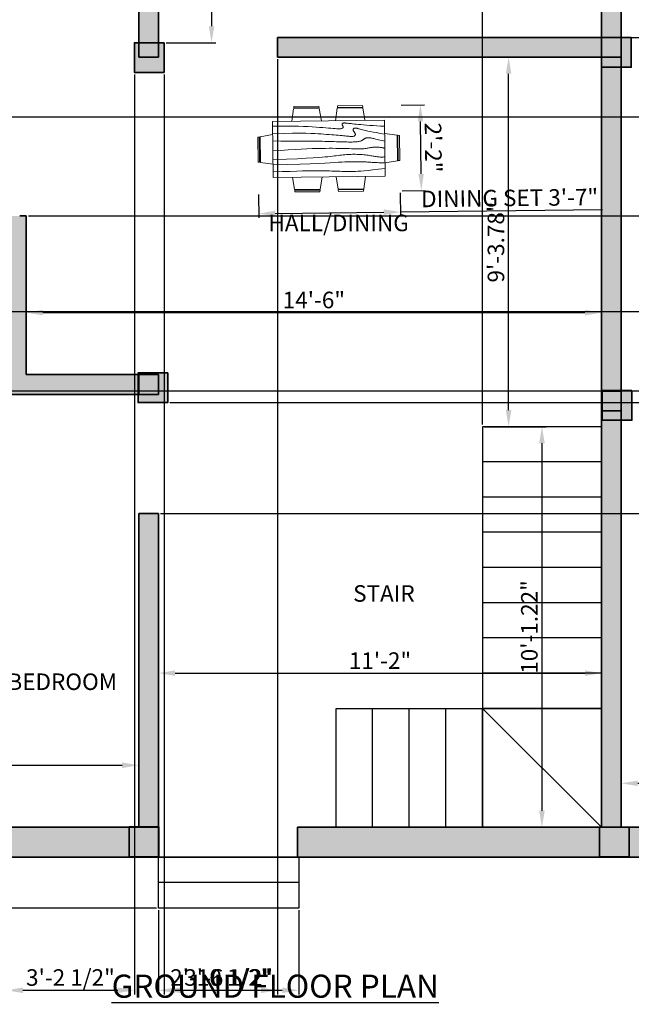
# Model space of a CAD drawing. Units: inches. Extents: x -36 to 490, y -420 to 94.
# Tile 2 of 4: x 99 to 284, y -420 to -122. Entities that reach past the tile are written whole.
import ezdxf

# ---------------------------------------------------------------- set-up
doc = ezdxf.new("R2010")
doc.units = ezdxf.units.IN
for name, color, linetype, lineweight in [('A-ANNO-DIMS', 2, 'Continuous', 18), ('A-ANNO-TEXT', 7, 'Continuous', 25), ('A-AREA-IDEN', 1, 'Continuous', 18), ('A-COLS', 1, 'Continuous', 35), ('A-FLOR-STRS', 3, 'Continuous', 25), ('A-WALL', 7, 'Continuous', 35), ('furn', 8, 'Continuous', 18)]:
    doc.layers.add(name, color=color, linetype=linetype, lineweight=lineweight)
doc.layers.add('A-WALL-PATT', color=177, linetype='Continuous', lineweight=13, true_color=0x293189)
doc.styles.get("Standard").update_dxf_attribs({"font": 'arial.ttf'})
doc.dimstyles.new('ISO-25', dxfattribs={"dimtxt": 5, "dimasz": 5, "dimexe": 1.25, "dimexo": 0.625, "dimtad": 1, "dimlunit": 3, "dimtxsty": 'Standard', "dimcen": 2.5, "dimadec": 0, "dimazin": 0, "dimtfac": 1, "dimtmove": 0, "dimatfit": 3, "dimfxl": 1, "dimarcsym": 0})

# ---------------------------------------------------------------- blocks, each defined once
blk = doc.blocks.new('*D1')
at = {"layer": 'A-ANNO-DIMS', "color": 0, "lineweight": -2, "transparency": 16777216}
for p, q in [((280.98, -352.29), (280.98, -351.67)), ((285.98, -352.92), (401.98, -352.92)), ((406.98, -352.29), (406.98, -351.67))]:
    blk.add_line(p, q, dxfattribs=at)
at = {"layer": 'A-ANNO-DIMS', "color": 0, "transparency": 16777216}
for points in [[(285.98, -352.09), (285.98, -353.75), (280.98, -352.92)], [(401.98, -352.09), (401.98, -353.75), (406.98, -352.92)]]:
    blk.add_solid(points, dxfattribs=at)
at = {"layer": 'Defpoints', "color": 0, "transparency": 16777216}
for p in [(280.98, -352.92), (406.98, -352.92), (406.98, -352.92)]:
    blk.add_point(p, dxfattribs=at)
at = {"layer": 'A-ANNO-DIMS', "color": 0, "transparency": 16777216, "insert": (343.98, -349.74), "char_height": 5, "attachment_point": 5}
blk.add_mtext('10\'-6"', dxfattribs=at)
blk = doc.blocks.new('*D3')
at = {"layer": 'A-ANNO-DIMS', "color": 0, "lineweight": -2, "transparency": 16777216}
for p, q in [((274.98, -309.55), (274.98, -320.83)), ((140.98, -319.35), (140.98, -320.83)), ((145.98, -319.58), (269.98, -319.58))]:
    blk.add_line(p, q, dxfattribs=at)
at = {"layer": 'A-ANNO-DIMS', "color": 0, "transparency": 16777216}
for points in [[(145.98, -318.74), (145.98, -320.41), (140.98, -319.58)], [(269.98, -318.74), (269.98, -320.41), (274.98, -319.58)]]:
    blk.add_solid(points, dxfattribs=at)
at = {"layer": 'Defpoints', "color": 0, "transparency": 16777216}
for p in [(274.98, -308.92), (140.98, -318.73), (274.98, -319.58)]:
    blk.add_point(p, dxfattribs=at)
at = {"layer": 'A-ANNO-DIMS', "color": 0, "transparency": 16777216, "insert": (207.98, -316.44), "char_height": 5, "attachment_point": 5}
blk.add_mtext('11\'-2"', dxfattribs=at)
blk = doc.blocks.new('*D4')
at = {"layer": 'A-ANNO-DIMS', "color": 0, "lineweight": -2, "transparency": 16777216}
for p, q in [((239.61, -245.01), (258.23, -245.01)), ((256.98, -250.01), (256.98, -361.23)), ((239.61, -366.23), (258.23, -366.23))]:
    blk.add_line(p, q, dxfattribs=at)
at = {"layer": 'A-ANNO-DIMS', "color": 0, "transparency": 16777216}
for points in [[(256.15, -250.01), (257.82, -250.01), (256.98, -245.01)], [(256.15, -361.23), (257.82, -361.23), (256.98, -366.23)]]:
    blk.add_solid(points, dxfattribs=at)
at = {"layer": 'Defpoints', "color": 0, "transparency": 16777216}
for p in [(238.98, -245.01), (238.98, -366.23), (256.98, -366.23)]:
    blk.add_point(p, dxfattribs=at)
at = {"layer": 'A-ANNO-DIMS', "color": 0, "transparency": 16777216, "insert": (253.81, -305.62), "char_height": 5, "attachment_point": 5, "rotation": 90}
blk.add_mtext('10\'-1.22"', dxfattribs=at)
blk = doc.blocks.new('*D5')
at = {"layer": 'A-ANNO-DIMS', "color": 0, "lineweight": -2, "transparency": 16777216}
for p, q in [((9.59, -330.42), (9.59, -348.7)), ((134.98, -330.42), (134.98, -348.7)), ((14.59, -347.45), (129.98, -347.45))]:
    blk.add_line(p, q, dxfattribs=at)
at = {"layer": 'A-ANNO-DIMS', "color": 0, "transparency": 16777216}
for points in [[(14.59, -346.62), (14.59, -348.29), (9.59, -347.45)], [(129.98, -346.62), (129.98, -348.29), (134.98, -347.45)]]:
    blk.add_solid(points, dxfattribs=at)
at = {"layer": 'Defpoints', "color": 0, "transparency": 16777216}
for p in [(9.59, -329.79), (134.98, -329.79), (134.98, -347.45)]:
    blk.add_point(p, dxfattribs=at)
at = {"layer": 'A-ANNO-DIMS', "color": 0, "transparency": 16777216, "insert": (72.29, -344.27), "char_height": 5, "attachment_point": 5}
blk.add_mtext('10\'-5.39"', dxfattribs=at)
blk = doc.blocks.new('*D14')
at = {"layer": 'A-ANNO-DIMS', "color": 0, "lineweight": -2, "transparency": 16777216}
for p, q in [((141.61, 4.77), (158.28, 4.77)), ((157.03, -0.23), (157.03, -123.83)), ((143.3, -128.83), (158.28, -128.83))]:
    blk.add_line(p, q, dxfattribs=at)
at = {"layer": 'A-ANNO-DIMS', "color": 0, "transparency": 16777216}
for points in [[(156.2, -0.23), (157.86, -0.23), (157.03, 4.77)], [(156.2, -123.83), (157.86, -123.83), (157.03, -128.83)]]:
    blk.add_solid(points, dxfattribs=at)
at = {"layer": 'Defpoints', "color": 0, "transparency": 16777216}
for p in [(140.98, 4.77), (142.67, -128.83), (157.03, -128.83)]:
    blk.add_point(p, dxfattribs=at)
at = {"layer": 'A-ANNO-DIMS', "color": 0, "transparency": 16777216, "insert": (153.85, -62.03), "char_height": 5, "attachment_point": 5, "rotation": 90}
blk.add_mtext('11\'-1.6"', dxfattribs=at)
blk = doc.blocks.new('*D15')
at = {"layer": 'A-ANNO-DIMS', "color": 0, "lineweight": -2, "transparency": 16777216}
for p, q in [((281.61, 2.85), (295.66, 2.85)), ((294.41, -2.15), (294.41, -122.23)), ((281.61, -127.23), (295.66, -127.23))]:
    blk.add_line(p, q, dxfattribs=at)
at = {"layer": 'A-ANNO-DIMS', "color": 0, "transparency": 16777216}
for points in [[(293.58, -2.15), (295.25, -2.15), (294.41, 2.85)], [(293.58, -122.23), (295.25, -122.23), (294.41, -127.23)]]:
    blk.add_solid(points, dxfattribs=at)
at = {"layer": 'Defpoints', "color": 0, "transparency": 16777216}
for p in [(280.98, 2.85), (280.98, -127.23), (294.41, -127.23)]:
    blk.add_point(p, dxfattribs=at)
at = {"layer": 'A-ANNO-DIMS', "color": 0, "transparency": 16777216, "insert": (291.24, -62.19), "char_height": 5, "attachment_point": 5, "rotation": 90}
blk.add_mtext('10\'-10.08"', dxfattribs=at)
blk = doc.blocks.new('*D17')
at = {"layer": 'A-ANNO-DIMS', "color": 0, "lineweight": -2, "transparency": 16777216}
for p, q in [((100.98, -209.87), (100.98, -209.25)), ((105.98, -210.5), (269.98, -210.5)), ((274.98, -209.87), (274.98, -209.25))]:
    blk.add_line(p, q, dxfattribs=at)
at = {"layer": 'A-ANNO-DIMS', "color": 0, "transparency": 16777216}
for points in [[(105.98, -209.66), (105.98, -211.33), (100.98, -210.5)], [(269.98, -209.66), (269.98, -211.33), (274.98, -210.5)]]:
    blk.add_solid(points, dxfattribs=at)
at = {"layer": 'Defpoints', "color": 0, "transparency": 16777216}
for p in [(100.98, -210.5), (274.98, -210.5), (274.98, -210.5)]:
    blk.add_point(p, dxfattribs=at)
at = {"layer": 'A-ANNO-DIMS', "color": 0, "transparency": 16777216, "insert": (187.98, -207.32), "char_height": 5, "attachment_point": 5}
blk.add_mtext('14\'-6"', dxfattribs=at)
blk = doc.blocks.new('*D18')
at = {"layer": 'A-ANNO-DIMS', "color": 0, "lineweight": -2, "transparency": 16777216}
for p, q in [((235.12, -133.23), (248.14, -133.23)), ((246.89, -240.01), (246.89, -138.23)), ((239.61, -245.01), (248.14, -245.01))]:
    blk.add_line(p, q, dxfattribs=at)
at = {"layer": 'A-ANNO-DIMS', "color": 0, "transparency": 16777216}
for points in [[(246.06, -138.23), (247.72, -138.23), (246.89, -133.23)], [(246.06, -240.01), (247.72, -240.01), (246.89, -245.01)]]:
    blk.add_solid(points, dxfattribs=at)
at = {"layer": 'Defpoints', "color": 0, "transparency": 16777216}
for p in [(234.5, -133.23), (246.89, -133.23), (238.98, -245.01)]:
    blk.add_point(p, dxfattribs=at)
at = {"layer": 'A-ANNO-DIMS', "color": 0, "transparency": 16777216, "insert": (243.71, -189.12), "char_height": 5, "attachment_point": 5, "rotation": 90}
blk.add_mtext('9\'-3.78"', dxfattribs=at)
blk = doc.blocks.new('Dining Set - 36 x 72 in.')
for p, q in [((-22.2343, 26.00059), (-23.4847, 17.99762)), ((-22.2304, 26), (-5.7608, 26)), ((-22, 27.5), (-22.1562, 26.50042)), ((-5.8416, 26.5), (-22.1534, 26.5)), ((-22, 27.5), (-6, 27.5)), ((-5.8437, 26.49966), (-6, 27.5)), ((-4.5152, 17.99762), (-5.7655, 25.99926)), ((5.7657, 26.00059), (4.5153, 17.99762)), ((5.7696, 26), (22.2392, 26)), ((6, 27.5), (5.8438, 26.50042)), ((22.1584, 26.5), (5.8466, 26.5)), ((6, 27.5), (22, 27.5)), ((22.1563, 26.49966), (22, 27.5)), ((23.4848, 17.99762), (22.2345, 25.99926)), ((36, 18), (-36, 18)), ((-36, 18), (-36, -18)), ((36, -18), (36, 18)), ((-45.5, 8), (-44.5004, 8.15617)), ((-45.5, 8), (-45.5, -8)), ((-44.5, -8.15843), (-44.5, 8.15338)), ((-44.0006, 8.23428), (-35.9976, 9.48474)), ((-44, 8.23041), (-44, -8.23915)), ((44.0006, 8.23428), (35.9976, 9.48474)), ((44, 8.23041), (44, -8.23915)), ((44.5, -8.15843), (44.5, 8.15338)), ((45.5, 8), (44.5005, 8.15617)), ((45.5, 8), (45.5, -8)), ((-44.4997, -8.15631), (-45.5, -8)), ((-35.9976, -9.48476), (-43.9993, -8.2345)), ((35.9976, -9.48476), (43.9993, -8.2345)), ((44.4997, -8.15631), (45.5, -8)), ((-36, -18), (36, -18)), ((-22.2343, -26.0006), (-23.4847, -17.99762)), ((-4.5152, -17.99762), (-5.7655, -25.99928)), ((5.7657, -26.0006), (4.5153, -17.99762)), ((23.4848, -17.99762), (22.2345, -25.99928)), ((-22.2304, -26), (-5.7608, -26)), ((-22, -27.5), (-22.1562, -26.50044)), ((-5.8416, -26.5), (-22.1534, -26.5)), ((-22, -27.5), (-6, -27.5)), ((-5.8437, -26.49967), (-6, -27.5)), ((5.7696, -26), (22.2392, -26)), ((6, -27.5), (5.8438, -26.50044)), ((22.1584, -26.5), (5.8466, -26.5)), ((6, -27.5), (22, -27.5)), ((22.1563, -26.49967), (22, -27.5))]:
    blk.add_line(p, q)
for points in [[(-36, 15), (-31.1772, 14.97754), (-26.8079, 14.91406), (-22.8538, 14.81543), (-19.276, 14.6875), (-16.0362, 14.53613), (-13.0957, 14.36718), (-10.4159, 14.18652), (-7.9583, 14), (-5.6904, 13.81315), (-3.6035, 13.63021), (-1.6954, 13.45508), (0.0365, 13.29166), (1.5945, 13.14388), (2.9811, 13.01562), (4.1988, 12.9108), (5.25, 12.83333), (6.1393, 12.78613), (6.8802, 12.76823), (7.4883, 12.77767), (7.9792, 12.8125), (8.3685, 12.87077), (8.6719, 12.95052), (8.9049, 13.0498), (9.0833, 13.16666), (9.2205, 13.29899), (9.3216, 13.44401), (9.3895, 13.59879), (9.4271, 13.76041), (9.4373, 13.92594), (9.4232, 14.09245), (9.3875, 14.257), (9.3333, 14.41666), (9.2638, 14.56917), (9.1836, 14.71484), (9.0975, 14.85465), (9.0104, 14.98958), (8.9272, 15.1206), (8.8529, 15.2487), (8.7922, 15.37483), (8.75, 15.5), (8.7305, 15.62467), (8.7344, 15.74739), (8.7617, 15.86621), (8.8125, 15.97916), (8.8867, 16.08431), (8.9844, 16.17968), (9.1055, 16.26334), (9.25, 16.33333), (9.4189, 16.38802), (9.6172, 16.42708), (9.8506, 16.45052), (10.125, 16.45833), (10.4463, 16.45052), (10.8203, 16.42708), (11.2529, 16.38802), (11.75, 16.33333), (12.3184, 16.26318), (12.9694, 16.17838), (13.7151, 16.07991), (14.5677, 15.96875), (15.5395, 15.84586), (16.6426, 15.71224), (17.8893, 15.56884), (19.2917, 15.41666), (20.859, 15.25667), (22.5879, 15.08984), (24.4721, 14.91715), (26.5052, 14.73958), (28.6809, 14.5581), (30.9929, 14.3737), (33.4347, 14.18733), (36, 14)], [(-36, 10), (-28.9766, 10.14274), (-23.1725, 10.20442), (-18.4241, 10.19775), (-14.5677, 10.13541), (-11.4399, 10.03011), (-8.877, 9.89453), (-6.7154, 9.74137), (-4.7917, 9.58333), (-2.9698, 9.43082), (-1.2246, 9.28515), (0.4415, 9.14534), (2.026, 9.01041), (3.5266, 8.87939), (4.9408, 8.7513), (6.266, 8.62516), (7.5, 8.5), (8.6411, 8.37549), (9.6914, 8.2539), (10.6538, 8.13818), (11.5312, 8.03125), (12.3267, 7.93603), (13.043, 7.85547), (13.6831, 7.79248), (14.25, 7.75), (14.7471, 7.7303), (15.1797, 7.73307), (15.5537, 7.75732), (15.875, 7.80208), (16.1494, 7.86637), (16.3828, 7.94922), (16.5811, 8.04964), (16.75, 8.16666), (16.8944, 8.29915), (17.0143, 8.44531), (17.1089, 8.60319), (17.1771, 8.77083), (17.218, 8.94629), (17.2305, 9.1276), (17.2137, 9.31282), (17.1667, 9.5), (17.0895, 9.6875), (16.987, 9.875), (16.8649, 10.0625), (16.7292, 10.25), (16.5856, 10.4375), (16.4401, 10.625), (16.2985, 10.8125), (16.1667, 11), (16.05, 11.18733), (15.9518, 11.3737), (15.8752, 11.5581), (15.8229, 11.73958), (15.798, 11.91715), (15.8034, 12.08984), (15.842, 12.25667), (15.9167, 12.41666), (16.0295, 12.56836), (16.1784, 12.70833), (16.3605, 12.83268), (16.5729, 12.9375), (16.8127, 13.01888), (17.0768, 13.07291), (17.3625, 13.0957), (17.6667, 13.08333), (17.9894, 13.03312), (18.3418, 12.94726), (18.7382, 12.82918), (19.1927, 12.68229), (19.7195, 12.51001), (20.3327, 12.31575), (21.0465, 12.10294), (21.875, 11.875), (22.8357, 11.63354), (23.959, 11.37304), (25.2786, 11.08618), (26.8282, 10.76562), (28.6414, 10.40405), (30.752, 9.99414), (33.1936, 9.52856), (36, 9)], [(-36, 5.5), (-30.7157, 5.3348), (-26.069, 5.20963), (-21.9946, 5.11767), (-18.4271, 5.05208), (-15.3009, 5.00602), (-12.5508, 4.97265), (-10.1112, 4.94515), (-7.9167, 4.91666), (-5.909, 4.88167), (-4.0586, 4.83984), (-2.3429, 4.79215), (-0.7396, 4.73958), (0.7739, 4.6831), (2.22, 4.6237), (3.6213, 4.56233), (5, 4.5), (6.373, 4.43782), (7.7344, 4.3776), (9.0723, 4.32129), (10.375, 4.27083), (11.6309, 4.22819), (12.8281, 4.19531), (13.9551, 4.17415), (15, 4.16666), (15.954, 4.17448), (16.819, 4.19791), (17.6001, 4.23698), (18.3021, 4.29166), (18.9299, 4.36198), (19.4883, 4.44791), (19.9823, 4.54948), (20.4167, 4.66666), (20.7969, 4.79899), (21.1302, 4.94401), (21.4245, 5.09879), (21.6875, 5.26041), (21.9271, 5.42594), (22.1511, 5.59245), (22.3672, 5.757), (22.5834, 5.91666), (22.8065, 6.06868), (23.0404, 6.21093), (23.2879, 6.34147), (23.5521, 6.45833), (23.8358, 6.55957), (24.142, 6.64323), (24.4735, 6.70735), (24.8334, 6.75), (25.2235, 6.76969), (25.642, 6.76692), (26.0858, 6.74267), (26.5521, 6.69791), (27.0379, 6.63362), (27.5404, 6.55078), (28.0565, 6.45036), (28.5834, 6.33333), (29.1242, 6.19987), (29.7071, 6.04687), (30.3661, 5.87044), (31.1354, 5.66666), (32.0493, 5.43164), (33.142, 5.16146), (34.4475, 4.85221), (36, 4.5)], [(-36, -1), (-30.7915, -0.6591), (-26.0195, -0.38216), (-21.6519, -0.16284), (-17.6563, 0.00521), (-14.0005, 0.12833), (-10.6523, 0.21289), (-7.5796, 0.26522), (-4.75, 0.29166), (-2.134, 0.29793), (0.2878, 0.28711), (2.5317, 0.26163), (4.6146, 0.22396), (6.5529, 0.17651), (8.3633, 0.12174), (10.0623, 0.06209), (11.6667, 0), (13.1899, -0.06201), (14.6341, -0.1211), (15.9982, -0.17432), (17.2813, -0.21875), (18.4823, -0.25147), (19.6003, -0.26953), (20.6343, -0.27002), (21.5834, -0.25), (22.4481, -0.20768), (23.2357, -0.14584), (23.9549, -0.06836), (24.6146, 0.02083), (25.2235, 0.11784), (25.7904, 0.21875), (26.3241, 0.31966), (26.8334, 0.41666), (27.3265, 0.50618), (27.8099, 0.58593), (28.2894, 0.65397), (28.7709, 0.70833), (29.2601, 0.74707), (29.763, 0.76823), (30.2855, 0.76985), (30.8334, 0.75), (31.4088, 0.70784), (31.9994, 0.64713), (32.589, 0.57275), (33.1615, 0.48958), (33.7008, 0.4025), (34.1908, 0.3164), (34.6153, 0.23616), (34.9584, 0.16666), (35.2099, 0.11165), (35.3848, 0.07031), (35.504, 0.04069), (35.5886, 0.02083), (35.6594, 0.00879), (35.7377, 0.0026), (35.8442, 0.00032), (36, 0)], [(-36, -6.5), (-27.1843, -6.31267), (-20.084, -6.1263), (-14.469, -5.9419), (-10.1094, -5.76042), (-6.7752, -5.58285), (-4.2363, -5.41016), (-2.2629, -5.24333), (-0.625, -5.08334), (0.8708, -4.93099), (2.2715, -4.78646), (3.5872, -4.64974), (4.8281, -4.52084), (6.0046, -4.39974), (7.127, -4.28646), (8.2053, -4.18099), (9.25, -4.08334), (10.2705, -3.99382), (11.2734, -3.91407), (12.2647, -3.84603), (13.25, -3.79167), (14.2354, -3.75293), (15.2266, -3.73177), (16.2295, -3.73015), (17.25, -3.75), (18.2912, -3.79248), (19.3451, -3.85547), (20.4009, -3.93604), (21.4479, -4.03125), (22.4754, -4.13819), (23.4727, -4.25391), (24.4289, -4.37549), (25.3334, -4.5), (26.1785, -4.62492), (26.9694, -4.74935), (27.7145, -4.87281), (28.4219, -4.99479), (29.1, -5.11483), (29.7572, -5.23242), (30.4016, -5.34709), (31.0417, -5.45834), (31.6837, -5.56437), (32.3262, -5.65821), (32.9658, -5.73153), (33.599, -5.77604), (34.2224, -5.78345), (34.8327, -5.74545), (35.4264, -5.65373), (36, -5.5)], [(-36, -10), (-26.4022, -9.81299), (-18.4675, -9.62891), (-11.9839, -9.45069), (-6.7396, -9.28125), (-2.5226, -9.12354), (0.8789, -8.98047), (3.6769, -8.85498), (6.0833, -8.75), (8.2767, -8.66765), (10.3021, -8.60677), (12.1712, -8.56543), (13.8958, -8.54167), (15.4876, -8.53353), (16.9583, -8.53907), (18.3197, -8.55632), (19.5834, -8.58334), (20.7616, -8.61841), (21.8685, -8.66081), (22.9188, -8.71004), (23.9271, -8.76563), (24.9081, -8.82707), (25.8763, -8.89388), (26.8465, -8.96558), (27.8334, -9.04167), (28.8474, -9.12118), (29.8828, -9.20117), (30.93, -9.27824), (31.9792, -9.34896), (33.0205, -9.40991), (34.0443, -9.45768), (35.0407, -9.48885), (36, -9.5)], [(-36, -14.5), (-30.0881, -14.33513), (-25.0332, -14.21224), (-20.7312, -14.12647), (-17.0781, -14.07292), (-13.97, -14.04671), (-11.3027, -14.04297), (-8.9724, -14.05681), (-6.875, -14.08334), (-4.9224, -14.11833), (-3.0905, -14.16016), (-1.3709, -14.20785), (0.2448, -14.26042), (1.7647, -14.3169), (3.1973, -14.3763), (4.5507, -14.43767), (5.8333, -14.5), (7.0554, -14.5621), (8.235, -14.62175), (9.3922, -14.67652), (10.5469, -14.72396), (11.7192, -14.76164), (12.929, -14.78711), (14.1965, -14.79794), (15.5417, -14.79167), (16.9933, -14.76424), (18.6152, -14.70508), (20.4804, -14.60197), (22.6615, -14.44271), (25.2312, -14.21509), (28.2624, -13.9069), (31.8277, -13.50594), (36, -13)]]:
    blk.add_lwpolyline(points)
blk = doc.blocks.new('COLUMN-9X9')
h = blk.add_hatch(color=256)
h.dxf.hatch_style = 1
h.paths.add_polyline_path([(9, 0), (9, 9), (0, 9), (0, 0)])
blk.add_lwpolyline([(0, 9), (9, 9), (9, 0), (0, 0)], close=True)
blk = doc.blocks.new('*D36')
at = {"layer": 'A-ANNO-DIMS', "color": 0, "lineweight": -2, "transparency": 16777216}
for p, q in [((171.21, -174.74), (171.29, -181.8)), ((214.06, -174.24), (214.14, -181.3)), ((176.27, -180.49), (209.13, -180.1)), ((214.13, -180.05), (275.33, -179.33))]:
    blk.add_line(p, q, dxfattribs=at)
at = {"layer": 'A-ANNO-DIMS', "color": 0, "transparency": 16777216}
for points in [[(176.26, -179.66), (176.28, -181.32), (171.27, -180.55)], [(209.12, -179.27), (209.14, -180.94), (214.13, -180.05)]]:
    blk.add_solid(points, dxfattribs=at)
at = {"layer": 'Defpoints', "color": 0, "transparency": 16777216}
for p in [(171.2, -174.12), (214.05, -173.62), (214.13, -180.05)]:
    blk.add_point(p, dxfattribs=at)
at = {"layer": 'A-ANNO-DIMS', "color": 0, "transparency": 16777216, "insert": (247.19, -176.45), "char_height": 5, "attachment_point": 5, "rotation": 0.6702}
blk.add_mtext('DINING SET 3\'-7"', dxfattribs=at)
blk = doc.blocks.new('*D37')
at = {"layer": 'A-ANNO-DIMS', "color": 0, "lineweight": -2, "transparency": 16777216}
for p, q in [((214.37, -147.71), (221.43, -147.63)), ((220.42, -168.54), (220.24, -152.64)), ((214.68, -173.61), (221.73, -173.53))]:
    blk.add_line(p, q, dxfattribs=at)
at = {"layer": 'A-ANNO-DIMS', "color": 0, "transparency": 16777216}
for points in [[(221.07, -152.63), (219.4, -152.65), (220.18, -147.64)], [(221.26, -168.53), (219.59, -168.55), (220.48, -173.54)]]:
    blk.add_solid(points, dxfattribs=at)
at = {"layer": 'Defpoints', "color": 0, "transparency": 16777216}
for p in [(213.75, -147.72), (220.18, -147.64), (214.05, -173.62)]:
    blk.add_point(p, dxfattribs=at)
at = {"layer": 'A-ANNO-DIMS', "color": 0, "transparency": 16777216, "insert": (223.46, -160.56), "char_height": 5, "attachment_point": 5, "rotation": 270.6702}
blk.add_mtext('2\'-2"', dxfattribs=at)
blk = doc.blocks.new('*D38')
at = {"layer": 'A-ANNO-DIMS', "color": 0, "lineweight": -2, "transparency": 16777216}
for p, q in [((94.98, -133.85), (94.98, -416.79)), ((133.67, -138.45), (133.67, -416.79)), ((99.98, -415.54), (128.67, -415.54))]:
    blk.add_line(p, q, dxfattribs=at)
at = {"layer": 'A-ANNO-DIMS', "color": 0, "transparency": 16777216}
for points in [[(99.98, -414.7), (99.98, -416.37), (94.98, -415.54)], [(128.67, -414.7), (128.67, -416.37), (133.67, -415.54)]]:
    blk.add_solid(points, dxfattribs=at)
at = {"layer": 'Defpoints', "color": 0, "transparency": 16777216}
for p in [(94.98, -133.23), (133.67, -137.83), (133.67, -415.54)]:
    blk.add_point(p, dxfattribs=at)
at = {"layer": 'A-ANNO-DIMS', "color": 0, "transparency": 16777216, "insert": (114.33, -412.32), "char_height": 5, "attachment_point": 5}
blk.add_mtext('3\'-2 1/2"', dxfattribs=at)
blk = doc.blocks.new('*D39')
at = {"layer": 'A-ANNO-DIMS', "color": 0, "lineweight": -2, "transparency": 16777216}
for p, q in [((238.98, -244.38), (238.98, 39.87)), ((274.98, -244.38), (274.98, 39.87)), ((243.98, 38.62), (269.98, 38.62))]:
    blk.add_line(p, q, dxfattribs=at)
at = {"layer": 'A-ANNO-DIMS', "color": 0, "transparency": 16777216}
for points in [[(243.98, 39.45), (243.98, 37.79), (238.98, 38.62)], [(269.98, 39.45), (269.98, 37.79), (274.98, 38.62)]]:
    blk.add_solid(points, dxfattribs=at)
at = {"layer": 'Defpoints', "color": 0, "transparency": 16777216}
for p in [(274.98, 38.62), (238.98, -245.01), (274.98, -245.01)]:
    blk.add_point(p, dxfattribs=at)
at = {"layer": 'A-ANNO-DIMS', "color": 0, "transparency": 16777216, "insert": (256.98, 41.8), "char_height": 5, "attachment_point": 5}
blk.add_mtext('3\'-0"', dxfattribs=at)
blk = doc.blocks.new('*D40')
at = {"layer": 'A-ANNO-DIMS', "color": 0, "lineweight": -2, "transparency": 16777216}
for p, q in [((140.98, -391.31), (140.98, -416.79)), ((183.4, -391.31), (183.4, -416.79)), ((145.98, -415.54), (178.4, -415.54))]:
    blk.add_line(p, q, dxfattribs=at)
at = {"layer": 'A-ANNO-DIMS', "color": 0, "transparency": 16777216}
for points in [[(145.98, -414.7), (145.98, -416.37), (140.98, -415.54)], [(178.4, -414.7), (178.4, -416.37), (183.4, -415.54)]]:
    blk.add_solid(points, dxfattribs=at)
at = {"layer": 'Defpoints', "color": 0, "transparency": 16777216}
for p in [(140.98, -390.69), (183.4, -390.69), (183.4, -415.54)]:
    blk.add_point(p, dxfattribs=at)
at = {"layer": 'A-ANNO-DIMS', "color": 0, "transparency": 16777216, "insert": (162.19, -412.32), "char_height": 5, "attachment_point": 5}
blk.add_mtext('3\'-6 1/2"', dxfattribs=at)
blk = doc.blocks.new('*D41')
at = {"layer": 'A-ANNO-DIMS', "color": 0, "lineweight": -2, "transparency": 16777216}
for p, q in [((326.36, -210.23), (-26.2, -210.23)), ((-24.95, -215.23), (-24.95, -229.23)), ((326.36, -234.23), (-26.2, -234.23))]:
    blk.add_line(p, q, dxfattribs=at)
at = {"layer": 'A-ANNO-DIMS', "color": 0, "transparency": 16777216}
for points in [[(-25.78, -215.23), (-24.12, -215.23), (-24.95, -210.23)], [(-25.78, -229.23), (-24.12, -229.23), (-24.95, -234.23)]]:
    blk.add_solid(points, dxfattribs=at)
at = {"layer": 'Defpoints', "color": 0, "transparency": 16777216}
for p in [(326.98, -210.23), (-24.95, -234.23), (326.98, -234.23)]:
    blk.add_point(p, dxfattribs=at)
at = {"layer": 'A-ANNO-DIMS', "color": 0, "transparency": 16777216, "insert": (-28.13, -222.23), "char_height": 5, "attachment_point": 5, "rotation": 90}
blk.add_mtext('2\'-0"', dxfattribs=at)
blk = doc.blocks.new('*D42')
at = {"layer": 'A-ANNO-DIMS', "color": 0, "lineweight": -2, "transparency": 16777216}
for p, q in [((-0.64, 13.77), (-26.2, 13.77)), ((-24.95, -385.69), (-24.95, 8.77)), ((140.36, -390.69), (-26.2, -390.69))]:
    blk.add_line(p, q, dxfattribs=at)
at = {"layer": 'A-ANNO-DIMS', "color": 0, "transparency": 16777216}
for points in [[(-25.78, 8.77), (-24.12, 8.77), (-24.95, 13.77)], [(-25.78, -385.69), (-24.12, -385.69), (-24.95, -390.69)]]:
    blk.add_solid(points, dxfattribs=at)
at = {"layer": 'Defpoints', "color": 0, "transparency": 16777216}
for p in [(-24.95, 13.77), (-0.02, 13.77), (140.98, -390.69)]:
    blk.add_point(p, dxfattribs=at)
at = {"layer": 'A-ANNO-DIMS', "color": 0, "transparency": 16777216, "insert": (-28.16, -188.46), "char_height": 5, "attachment_point": 5, "rotation": 90}
blk.add_mtext('33\'-8 1/2"', dxfattribs=at)
blk = doc.blocks.new('*D43')
at = {"layer": 'A-ANNO-DIMS', "color": 0, "lineweight": -2, "transparency": 16777216}
for p, q in [((176.98, -133.85), (176.98, -416.79)), ((142.67, -138.45), (142.67, -416.79)), ((147.67, -415.54), (171.98, -415.54))]:
    blk.add_line(p, q, dxfattribs=at)
at = {"layer": 'A-ANNO-DIMS', "color": 0, "transparency": 16777216}
for points in [[(147.67, -414.7), (147.67, -416.37), (142.67, -415.54)], [(171.98, -414.7), (171.98, -416.37), (176.98, -415.54)]]:
    blk.add_solid(points, dxfattribs=at)
at = {"layer": 'Defpoints', "color": 0, "transparency": 16777216}
for p in [(176.98, -133.23), (142.67, -137.83), (176.98, -415.54)]:
    blk.add_point(p, dxfattribs=at)
at = {"layer": 'A-ANNO-DIMS', "color": 0, "transparency": 16777216, "insert": (159.83, -412.32), "char_height": 5, "attachment_point": 5}
blk.add_mtext('2\'-10 1/2"', dxfattribs=at)
blk = doc.blocks.new('*D45')
at = {"layer": 'A-ANNO-DIMS', "color": 0, "lineweight": -2, "transparency": 16777216}
for p, q in [((95.61, -151.23), (442.2, -151.23)), ((440.95, -156.23), (440.95, -176.23)), ((101.61, -181.23), (442.2, -181.23))]:
    blk.add_line(p, q, dxfattribs=at)
at = {"layer": 'A-ANNO-DIMS', "color": 0, "transparency": 16777216}
for points in [[(440.11, -156.23), (441.78, -156.23), (440.95, -151.23)], [(440.11, -176.23), (441.78, -176.23), (440.95, -181.23)]]:
    blk.add_solid(points, dxfattribs=at)
at = {"layer": 'Defpoints', "color": 0, "transparency": 16777216}
for p in [(94.98, -151.23), (100.98, -181.23), (440.95, -181.23)]:
    blk.add_point(p, dxfattribs=at)
at = {"layer": 'A-ANNO-DIMS', "color": 0, "transparency": 16777216, "insert": (437.77, -166.23), "char_height": 5, "attachment_point": 5, "rotation": 90}
blk.add_mtext('2\'-6"', dxfattribs=at)
blk = doc.blocks.new('*D47')
at = {"layer": 'A-ANNO-DIMS', "color": 0, "lineweight": -2, "transparency": 16777216}
for p, q in [((144.42, -237.73), (442.2, -237.73)), ((440.95, -242.73), (440.95, -266.23)), ((141.61, -271.23), (442.2, -271.23))]:
    blk.add_line(p, q, dxfattribs=at)
at = {"layer": 'A-ANNO-DIMS', "color": 0, "transparency": 16777216}
for points in [[(440.11, -242.73), (441.78, -242.73), (440.95, -237.73)], [(440.11, -266.23), (441.78, -266.23), (440.95, -271.23)]]:
    blk.add_solid(points, dxfattribs=at)
at = {"layer": 'Defpoints', "color": 0, "transparency": 16777216}
for p in [(143.79, -237.73), (140.98, -271.23), (440.95, -271.23)]:
    blk.add_point(p, dxfattribs=at)
at = {"layer": 'A-ANNO-DIMS', "color": 0, "transparency": 16777216, "insert": (437.74, -254.48), "char_height": 5, "attachment_point": 5, "rotation": 90}
blk.add_mtext('2\'-9 1/2"', dxfattribs=at)

msp = doc.modelspace()

# ---------------------------------------------------------------- hatches: boundary and pattern name
at = {"layer": 'A-WALL-PATT'}
h = msp.add_hatch(color=256, dxfattribs=at)
h.dxf.hatch_style = 1
h.paths.add_polyline_path([(132.114, 13.772), (8.901, 13.772), (8.901, 4.772), (132.114, 4.772)])
h.paths.add_polyline_path([(274.98, 13.772), (141.114, 13.772), (141.114, 4.772), (274.98, 4.772)])
h.paths.add_polyline_path([(407.097, 13.772), (283.98, 13.772), (283.98, 4.772), (407.097, 4.772)])
h.paths.add_polyline_path([(280.984, 4.772), (274.984, 4.772), (274.984, -127.228), (280.984, -127.228)])
h.paths.add_polyline_path([(274.984, -127.228), (176.984, -127.228), (176.984, -133.228), (274.984, -133.228)])
h.paths.add_polyline_path([(140.984, 4.772), (134.984, 4.772), (134.984, -128.829), (140.984, -128.829)])
h.paths.add_polyline_path([(8.984, 4.772), (8.901, 4.772), (-0.016, 4.772), (-0.016, -127.003), (8.984, -127.003)])
h.paths.add_polyline_path([(94.984, -127.228), (8.984, -127.228), (8.984, -133.228), (88.984, -133.228), (88.984, -151.228), (94.984, -151.228), (94.984, -133.228)])
h.paths.add_polyline_path([(8.984, -136.003), (-0.016, -136.003), (-0.016, -228.965), (8.984, -228.965)])
h.paths.add_polyline_path([(100.984, -181.228), (98.984, -181.228), (88.984, -181.228), (8.984, -181.228), (8.984, -187.228), (88.984, -187.228), (94.984, -187.228), (94.984, -235.228), (134.793, -235.228), (134.793, -229.228), (100.984, -229.228)])
h.paths.add_polyline_path([(64.984, -229.228), (9.003, -229.228), (9.003, -235.228), (64.984, -235.228)], flags=17)
h.paths.add_polyline_path([(8.984, -237.965), (-0.016, -237.965), (-0.016, -366.285), (8.984, -366.285)])
h.paths.add_polyline_path([(132.054, -366.228), (9.018, -366.228), (9.018, -375.228), (132.054, -375.228)])
h.paths.add_polyline_path([(140.984, -271.228), (134.984, -271.228), (134.984, -366.131), (140.984, -366.131)])
h = msp.add_hatch(color=256, dxfattribs=at)
h.dxf.hatch_style = 1
h.paths.add_polyline_path([(280.984, -136.244), (274.984, -136.244), (274.984, -234.05), (280.984, -234.05)])
h.paths.add_polyline_path([(406.984, -127.228), (316.984, -127.228), (316.984, -133.228), (406.984, -133.228)])
h.paths.add_polyline_path([(415.984, 4.772), (406.984, 4.772), (406.984, -126.964), (415.984, -126.964)])
h = msp.add_hatch(color=256, dxfattribs=at)
h.dxf.hatch_style = 1
h.paths.add_polyline_path([(407.094, -366.228), (283.341, -366.228), (283.341, -375.228), (407.094, -375.228)])
h.paths.add_polyline_path([(415.984, -243.15), (406.984, -243.15), (406.984, -366.196), (415.984, -366.196)])
h.paths.add_polyline_path([(280.984, -243.05), (274.984, -243.05), (274.984, -366.161), (280.984, -366.161)])
h.paths.add_polyline_path([(274.341, -366.228), (182.984, -366.228), (182.984, -375.228), (183.401, -375.228), (274.341, -375.228)])

# ---------------------------------------------------------------- linework, layer by layer
at = {"layer": 'A-FLOR-STRS'}
for p, q in [((274.984, -245.007), (238.984, -245.007)), ((238.984, -245.007), (238.984, -366.228)), ((274.984, -255.66), (238.984, -255.66)), ((274.984, -266.313), (238.984, -266.313)), ((274.984, -276.965), (238.984, -276.965)), ((274.984, -287.618), (238.984, -287.618)), ((274.984, -298.271), (238.984, -298.271)), ((274.984, -308.923), (238.984, -308.923)), ((274.984, -319.576), (238.984, -319.576)), ((194.685, -366.228), (194.685, -330.228)), ((194.685, -330.228), (274.984, -330.228)), ((205.76, -366.228), (205.76, -330.228)), ((216.834, -366.228), (216.834, -330.228)), ((227.909, -366.228), (227.909, -330.228)), ((238.984, -330.228), (274.984, -366.228)), ((238.984, -366.228), (238.984, -330.228)), ((274.984, -330.228), (238.984, -330.228)), ((183.401, -382.957), (140.984, -382.957))]:
    msp.add_line(p, q, dxfattribs=at)
msp.add_lwpolyline([(140.984, -375.228), (183.401, -375.228), (183.401, -390.685), (140.984, -390.685)], close=True, dxfattribs=at)
at = {"layer": 'A-WALL'}
for p, q in [((134.984, -133.228), (134.984, 4.772)), ((140.984, -133.228), (140.984, 4.772)), ((274.984, -366.228), (274.984, 4.772)), ((280.984, -366.228), (280.984, 4.772)), ((176.984, -127.228), (274.984, -127.228)), ((176.984, -127.228), (176.984, -133.228)), ((274.984, -127.228), (280.984, -127.228)), ((134.984, -133.228), (140.984, -133.228)), ((176.984, -133.228), (274.984, -133.228)), ((274.984, -133.228), (280.984, -133.228)), ((98.984, -181.228), (100.984, -181.228)), ((100.984, -181.228), (100.984, -229.228)), ((100.984, -229.228), (134.984, -229.228)), ((134.984, -229.228), (140.984, -229.228)), ((134.984, -235.228), (134.984, -229.228)), ((140.984, -235.228), (140.984, -229.228)), ((94.984, -235.228), (134.984, -235.228)), ((134.984, -235.228), (140.984, -235.228)), ((280.984, -234.228), (274.984, -234.228)), ((280.984, -240.228), (274.984, -240.228)), ((134.984, -366.228), (134.984, -271.228)), ((134.984, -271.228), (140.984, -271.228)), ((140.984, -366.228), (140.984, -271.228)), ((140.984, -366.228), (8.984, -366.228)), ((140.984, -366.228), (140.984, -375.228)), ((182.984, -366.228), (182.984, -375.228)), ((274.984, -366.228), (182.984, -366.228)), ((406.984, -366.228), (274.984, -366.228))]:
    msp.add_line(p, q, dxfattribs=at)
msp.add_lwpolyline([(-0.016, 13.772), (415.984, 13.772), (415.984, -375.228), (-0.016, -375.228)], close=True, dxfattribs=at)

# ---------------------------------------------------------------- block references
at = {"layer": 'A-COLS'}
for p, rotation in [((275.009, -127.244), 270.0000000000002), ((133.674, -128.829), 270), ((134.793, -228.727), 269.9999999999994), ((275.178, -234.05), 269.9999999999997), ((132.054, -366.131), 269.9999999999994), ((274.34, -366.161), 270)]:
    msp.add_blockref('COLUMN-9X9', p, dxfattribs=dict(at, rotation=rotation))
at = {"layer": 'furn', "xscale": 0.4709428986025235, "yscale": 0.4709428986025235, "zscale": 0.4709428986025235, "rotation": 0.6701600822881935}
msp.add_blockref('Dining Set - 36 x 72 in.', (192.474, -160.919), dxfattribs=at)

# ---------------------------------------------------------------- texts
at = {"layer": 'A-ANNO-TEXT', "insert": (126.8, -410.795), "char_height": 7, "attachment_point": 1}
msp.add_mtext_dynamic_manual_height_columns('{\\LGROUND FLOOR PLAN}', width=277.08552, gutter_width=12.5, heights=[0], dxfattribs=at)
at = {"layer": 'A-AREA-IDEN', "char_height": 5, "attachment_point": 1}
for s, width, insert in [('{HALL/DINING}', 71.66616, (174.238, -180.865)), ('{STAIR}', 41.5854, (199.856, -292.973)), ('{BEDROOM}', 15.30121, (95.268, -319.675))]:
    msp.add_mtext_dynamic_manual_height_columns(s, width=width, gutter_width=12.5, heights=[0], dxfattribs=dict(at, insert=insert))

# ---------------------------------------------------------------- dimensions: what is measured, and where the dimension line sits
at = {"layer": 'A-ANNO-DIMS'}
for base, p1, p2, override, picture, middle in [((274.984, 38.622), (238.984, -245.007), (274.984, -245.007), {"dimdec": 1, "dimlfac": 1, "dimrnd": 0, "dimzin": 1, "dimdsep": 46, "dimlunit": 4, "dimfrac": 2}, '*D39', (256.984, 41.801)), ((133.675, -415.535), (94.984, -133.228), (133.675, -137.829), {"dimdec": 1, "dimlfac": 1, "dimrnd": 0, "dimzin": 1, "dimdsep": 46, "dimlunit": 4, "dimfrac": 2}, '*D38', (114.33, -412.323)), ((176.984, -415.535), (142.675, -137.829), (176.984, -133.228), {"dimdec": 1, "dimlfac": 1, "dimrnd": 0, "dimzin": 1, "dimdsep": 46, "dimlunit": 4, "dimfrac": 2}, '*D43', (159.83, -412.325)), ((274.984, -210.496), (100.984, -210.496), (274.984, -210.496), {"dimclrd": 0, "dimclre": 0, "dimclrt": 0}, '*D17', (187.984, -207.318)), ((274.984, -319.576), (140.984, -318.728), (274.984, -308.923), {"dimclrd": 0, "dimclre": 0, "dimclrt": 0}, '*D3', (207.984, -316.441)), ((134.984, -347.452), (9.595, -329.792), (134.984, -329.792), {"dimclrd": 0, "dimclre": 0, "dimclrt": 0}, '*D5', (72.289, -344.273)), ((406.984, -352.92), (280.984, -352.92), (406.984, -352.92), {"dimclrd": 0, "dimclre": 0, "dimclrt": 0}, '*D1', (343.984, -349.742)), ((183.401, -415.535), (140.984, -390.685), (183.401, -390.685), {"dimdec": 1, "dimlfac": 1, "dimrnd": 0, "dimzin": 1, "dimdsep": 46, "dimlunit": 4, "dimfrac": 2}, '*D40', (162.193, -412.323))]:
    dim = msp.add_linear_dim(base=base, p1=p1, p2=p2, dimstyle='ISO-25', override=override, dxfattribs=at)
    dim.commit()
    dim.dimension.update_dxf_attribs({"geometry": picture, "text_midpoint": middle})
for base, p1, p2, angle, override, picture, middle in [((-24.949, 13.772), (140.984, -390.685), (-0.016, 13.772), 90, {"dimdec": 1, "dimlfac": 1, "dimrnd": 0, "dimzin": 1, "dimdsep": 46, "dimlunit": 4, "dimfrac": 2}, '*D42', (-28.161, -188.457)), ((157.031, -128.829), (140.984, 4.772), (142.675, -128.829), 90, {"dimclrd": 0, "dimclre": 0, "dimclrt": 0}, '*D14', (153.853, -62.029)), ((294.414, -127.228), (280.984, 2.849), (280.984, -127.228), 90, {"dimclrd": 0, "dimclre": 0, "dimclrt": 0}, '*D15', (291.236, -62.19)), ((246.892, -133.228), (238.984, -245.007), (234.495, -133.228), 90, {"dimclrd": 0, "dimclre": 0, "dimclrt": 0}, '*D18', (243.712, -189.118)), ((220.177, -147.643), (214.052, -173.618), (213.749, -147.718), 90.67016, {"dimdec": 1, "dimlfac": 1, "dimrnd": 0, "dimzin": 1, "dimdsep": 46, "dimlunit": 4, "dimfrac": 2}, '*D37', (223.464, -160.556)), ((440.947, -181.228), (94.984, -151.228), (100.984, -181.228), 90, {"dimdec": 1, "dimlfac": 1, "dimrnd": 0, "dimzin": 1, "dimdsep": 46, "dimlunit": 4, "dimfrac": 2}, '*D45', (437.769, -166.228)), ((-24.949, -234.228), (326.984, -210.228), (326.984, -234.228), 90, {"dimdec": 1, "dimlfac": 1, "dimrnd": 0, "dimzin": 1, "dimdsep": 46, "dimlunit": 4, "dimfrac": 2}, '*D41', (-28.126, -222.228)), ((440.947, -271.228), (143.793, -237.727), (140.984, -271.228), 90, {"dimdec": 1, "dimlfac": 1, "dimrnd": 0, "dimzin": 1, "dimdsep": 46, "dimlunit": 4, "dimfrac": 2}, '*D47', (437.737, -254.478)), ((256.984, -366.228), (238.984, -245.007), (238.984, -366.228), 90, {"dimclrd": 0, "dimclre": 0, "dimclrt": 0}, '*D4', (253.806, -305.618))]:
    dim = msp.add_linear_dim(base=base, p1=p1, p2=p2, angle=angle, dimstyle='ISO-25', override=override, dxfattribs=at)
    dim.commit()
    dim.dimension.update_dxf_attribs({"geometry": picture, "text_midpoint": middle})
dim = msp.add_linear_dim(base=(214.128, -180.046), p1=(171.2, -174.119), p2=(214.052, -173.618), angle=0.67016, text='DINING SET <>', dimstyle='ISO-25', override={"dimdec": 1, "dimlfac": 1, "dimrnd": 0, "dimzin": 1, "dimdsep": 46, "dimlunit": 4, "dimfrac": 2}, dxfattribs=at)
dim.commit()
dim.dimension.update_dxf_attribs({"geometry": '*D36', "text_midpoint": (247.191, -176.447)})

doc.saveas('drawing.dxf')
